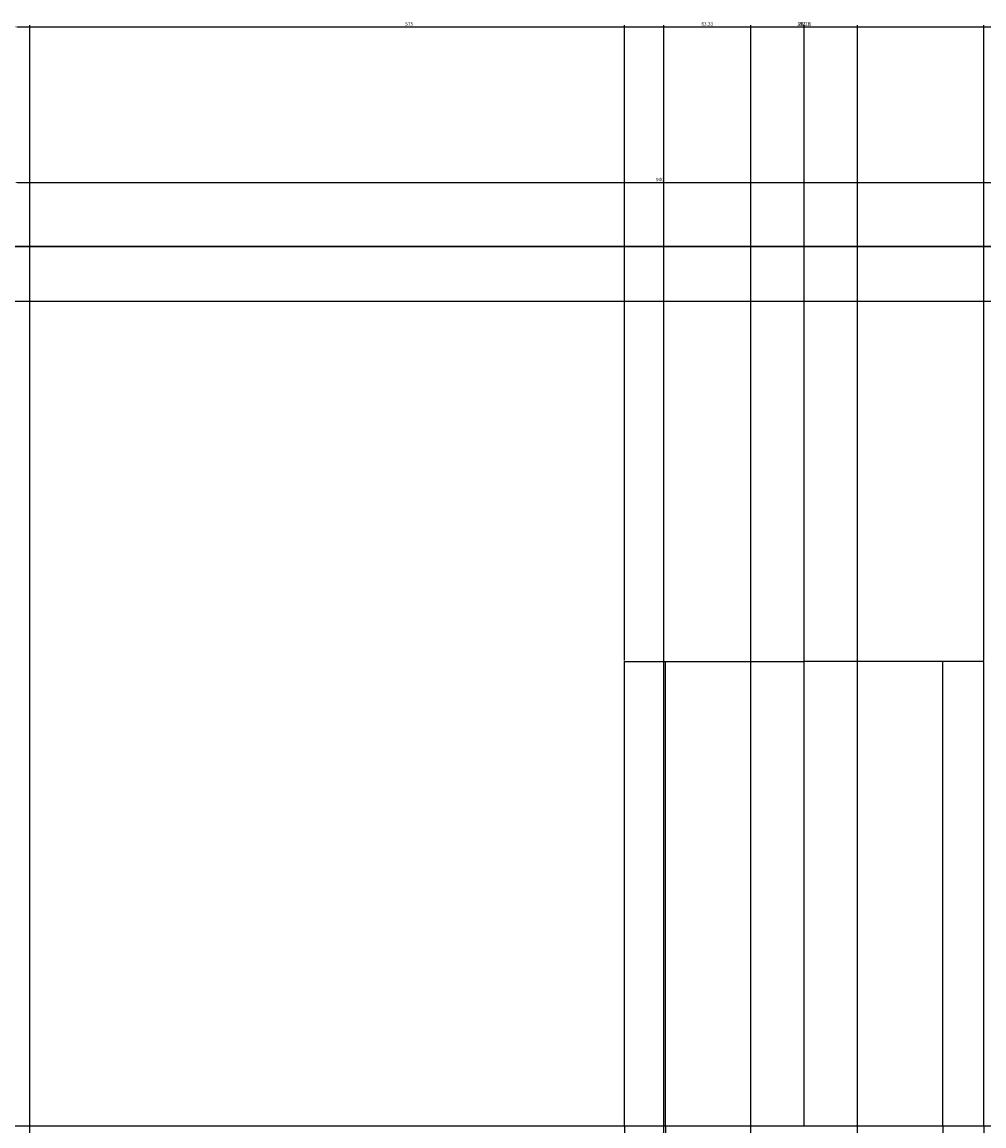
# Model space of a CAD drawing. Units: millimetres. Extents: x 2332 to 5836, y -853 to 2199.
# Tile 12 of 16: x 3641 to 4341, y 1368 to 2171. Entities that reach past the tile are written whole.
import ezdxf

# ---------------------------------------------------------------- set-up
doc = ezdxf.new("R2010")
doc.units = ezdxf.units.MM
for name, color, linetype, lineweight in [('A-ANNO-DIMS', 2, 'Continuous', 18), ('A-EQPM', 7, 'Continuous', 25), ('A-WALL', 8, 'Continuous', 30), ('SHELF', 40, 'Continuous', 25)]:
    doc.layers.add(name, color=color, linetype=linetype, lineweight=lineweight)
doc.styles.get("Standard").update_dxf_attribs({"font": 'arial.ttf'})
doc.dimstyles.new('ISO-25', dxfattribs={"dimtxt": 2.5, "dimasz": 2.5, "dimexe": 1.25, "dimexo": 0.625, "dimtad": 1, "dimtxsty": 'Standard', "dimcen": 2.5, "dimadec": 0, "dimazin": 0, "dimtfac": 1, "dimtmove": 0, "dimatfit": 3, "dimfxl": 1, "dimarcsym": 0})

# ---------------------------------------------------------------- blocks, each defined once
blk = doc.blocks.new('*D4')
at = {"layer": 'A-ANNO-DIMS', "color": 0, "lineweight": -2, "transparency": 16777216}
for p, q in [((3635.04, 2008.43), (3635.04, 2055.5)), ((3637.54, 2054.25), (4572.54, 2054.25)), ((4575.04, 2008.43), (4575.04, 2055.5))]:
    blk.add_line(p, q, dxfattribs=at)
at = {"layer": 'A-ANNO-DIMS', "color": 0, "transparency": 16777216}
for points in [[(3637.54, 2054.66), (3637.54, 2053.83), (3635.04, 2054.25)], [(4572.54, 2054.66), (4572.54, 2053.83), (4575.04, 2054.25)]]:
    blk.add_solid(points, dxfattribs=at)
at = {"layer": 'Defpoints', "color": 0, "transparency": 16777216}
for p in [(4575.04, 2054.25), (3635.04, 2007.8), (4575.04, 2007.8)]:
    blk.add_point(p, dxfattribs=at)
at = {"layer": 'A-ANNO-DIMS', "color": 0, "transparency": 16777216, "insert": (4105.04, 2056.15), "char_height": 2.5, "attachment_point": 5}
blk.add_mtext('940', dxfattribs=at)
blk = doc.blocks.new('*D23')
at = {"layer": 'A-ANNO-DIMS', "color": 0, "lineweight": -2, "transparency": 16777216}
for p, q in [((3646.47, 1030.43), (3646.47, 2168.7)), ((4773.61, 1030.43), (4773.61, 2168.7)), ((3648.97, 2167.45), (4771.11, 2167.45))]:
    blk.add_line(p, q, dxfattribs=at)
at = {"layer": 'A-ANNO-DIMS', "color": 0, "transparency": 16777216}
for points in [[(3648.97, 2167.87), (3648.97, 2167.04), (3646.47, 2167.45)], [(4771.11, 2167.87), (4771.11, 2167.04), (4773.61, 2167.45)]]:
    blk.add_solid(points, dxfattribs=at)
at = {"layer": 'Defpoints', "color": 0, "transparency": 16777216}
for p in [(4773.61, 2167.45), (3646.47, 1029.8), (4773.61, 1029.8)]:
    blk.add_point(p, dxfattribs=at)
at = {"layer": 'A-ANNO-DIMS', "color": 0, "transparency": 16777216, "insert": (4210.04, 2169.33), "char_height": 2.5, "attachment_point": 5}
blk.add_mtext('1127.1', dxfattribs=at)
blk = doc.blocks.new('*D24')
at = {"layer": 'A-ANNO-DIMS', "color": 0, "lineweight": -2, "transparency": 16777216}
for p, q in [((4079.19, 1706.43), (4079.19, 2168.7)), ((4340.89, 1706.43), (4340.89, 2168.7)), ((4081.69, 2167.45), (4338.39, 2167.45))]:
    blk.add_line(p, q, dxfattribs=at)
at = {"layer": 'A-ANNO-DIMS', "color": 0, "transparency": 16777216}
for points in [[(4081.69, 2167.87), (4081.69, 2167.04), (4079.19, 2167.45)], [(4338.39, 2167.87), (4338.39, 2167.04), (4340.89, 2167.45)]]:
    blk.add_solid(points, dxfattribs=at)
at = {"layer": 'Defpoints', "color": 0, "transparency": 16777216}
for p in [(4340.89, 2167.45), (4079.19, 1705.81), (4340.89, 1705.81)]:
    blk.add_point(p, dxfattribs=at)
at = {"layer": 'A-ANNO-DIMS', "color": 0, "transparency": 16777216, "insert": (4210.04, 2169.35), "char_height": 2.5, "attachment_point": 5}
blk.add_mtext('261.7', dxfattribs=at)
blk = doc.blocks.new('*D30')
at = {"layer": 'A-ANNO-DIMS', "color": 0, "lineweight": -2, "transparency": 16777216}
for p, q in [((3635.04, 1368.43), (3635.04, 2168.7)), ((4210.04, 1368.43), (4210.04, 2168.7)), ((3637.54, 2167.45), (4207.54, 2167.45))]:
    blk.add_line(p, q, dxfattribs=at)
at = {"layer": 'A-ANNO-DIMS', "color": 0, "transparency": 16777216}
for points in [[(3637.54, 2167.87), (3637.54, 2167.04), (3635.04, 2167.45)], [(4207.54, 2167.87), (4207.54, 2167.04), (4210.04, 2167.45)]]:
    blk.add_solid(points, dxfattribs=at)
at = {"layer": 'Defpoints', "color": 0, "transparency": 16777216}
for p in [(4210.04, 2167.45), (3635.04, 1367.8), (4210.04, 1367.8)]:
    blk.add_point(p, dxfattribs=at)
at = {"layer": 'A-ANNO-DIMS', "color": 0, "transparency": 16777216, "insert": (3922.54, 2169.35), "char_height": 2.5, "attachment_point": 5}
blk.add_mtext('575', dxfattribs=at)
blk = doc.blocks.new('*D31')
at = {"layer": 'A-ANNO-DIMS', "color": 0, "lineweight": -2, "transparency": 16777216}
for p, q in [((4171.16, 1017.67), (4171.16, 2168.7)), ((4248.92, 1017.67), (4248.92, 2168.7)), ((4173.66, 2167.45), (4246.42, 2167.45))]:
    blk.add_line(p, q, dxfattribs=at)
at = {"layer": 'A-ANNO-DIMS', "color": 0, "transparency": 16777216}
for points in [[(4173.66, 2167.87), (4173.66, 2167.04), (4171.16, 2167.45)], [(4246.42, 2167.87), (4246.42, 2167.04), (4248.92, 2167.45)]]:
    blk.add_solid(points, dxfattribs=at)
at = {"layer": 'Defpoints', "color": 0, "transparency": 16777216}
for p in [(4248.92, 2167.45), (4171.16, 1017.04), (4248.92, 1017.04)]:
    blk.add_point(p, dxfattribs=at)
at = {"layer": 'A-ANNO-DIMS', "color": 0, "transparency": 16777216, "insert": (4210.04, 2169.35), "char_height": 2.5, "attachment_point": 5}
blk.add_mtext('77.75', dxfattribs=at)
blk = doc.blocks.new('*D32')
at = {"layer": 'A-ANNO-DIMS', "color": 0, "lineweight": -2, "transparency": 16777216}
for p, q in [((4107.84, 1017.67), (4107.84, 2168.7)), ((4171.16, 1017.67), (4171.16, 2168.7)), ((4110.34, 2167.45), (4168.66, 2167.45))]:
    blk.add_line(p, q, dxfattribs=at)
at = {"layer": 'A-ANNO-DIMS', "color": 0, "transparency": 16777216}
for points in [[(4110.34, 2167.87), (4110.34, 2167.04), (4107.84, 2167.45)], [(4168.66, 2167.87), (4168.66, 2167.04), (4171.16, 2167.45)]]:
    blk.add_solid(points, dxfattribs=at)
at = {"layer": 'Defpoints', "color": 0, "transparency": 16777216}
for p in [(4171.16, 2167.45), (4107.84, 1017.04), (4171.16, 1017.04)]:
    blk.add_point(p, dxfattribs=at)
at = {"layer": 'A-ANNO-DIMS', "color": 0, "transparency": 16777216, "insert": (4139.5, 2169.36), "char_height": 2.5, "attachment_point": 5}
blk.add_mtext('63.33', dxfattribs=at)

msp = doc.modelspace()

# ---------------------------------------------------------------- linework, layer by layer
at = {"layer": 'A-EQPM'}
for p, q in [((4079.186, 1367.803), (4079.186, 1705.805)), ((4079.186, 1705.805), (4210.04, 1705.805)), ((4109.186, 1367.803), (4109.186, 1705.805)), ((4340.894, 1705.805), (4210.04, 1705.805)), ((4310.894, 1367.803), (4310.894, 1705.805)), ((4340.894, 1367.803), (4340.894, 1705.805)), ((4079.186, 1367.803), (4079.186, 1029.801)), ((4109.186, 1367.803), (4109.186, 1029.801)), ((4310.894, 1367.803), (4310.894, 1029.801)), ((4340.894, 1367.803), (4340.894, 1029.801))]:
    msp.add_line(p, q, dxfattribs=at)
at = {"layer": 'A-WALL'}
msp.add_line((3635.04, 2007.803), (4575.04, 2007.803), dxfattribs=at)
at = {"layer": 'SHELF'}
for p, q in [((3095.04, 1967.803), (4785.04, 1967.803)), ((4210.04, 1367.803), (4210.04, 1967.803)), ((3635.04, 1367.803), (4785.04, 1367.803))]:
    msp.add_line(p, q, dxfattribs=at)

# ---------------------------------------------------------------- dimensions: what is measured, and where the dimension line sits
at = {"layer": 'A-ANNO-DIMS'}
for base, p1, p2, override, picture, middle in [((4210.04, 2167.453), (3635.04, 1367.803), (4210.04, 1367.803), {"dimdec": 0, "dimlfac": 1, "dimrnd": 0, "dimzin": 0, "dimdsep": 46, "dimlunit": 2}, '*D30', (3922.54, 2169.35)), ((4773.612, 2167.453), (3646.468, 1029.801), (4773.612, 1029.801), {"dimdec": 1, "dimlfac": 1, "dimrnd": 0, "dimzin": 0, "dimdsep": 46, "dimlunit": 2}, '*D23', (4210.04, 2169.334)), ((4340.894, 2167.453), (4079.186, 1705.805), (4340.894, 1705.805), {"dimdec": 1, "dimlfac": 1, "dimrnd": 0, "dimzin": 0, "dimdsep": 46, "dimlunit": 2}, '*D24', (4210.04, 2169.355)), ((4171.163, 2167.453), (4107.837, 1017.045), (4171.163, 1017.045), {"dimdec": 2, "dimlfac": 1, "dimrnd": 0, "dimzin": 0, "dimdsep": 46, "dimlunit": 2}, '*D32', (4139.5, 2169.356)), ((4248.917, 2167.453), (4171.163, 1017.045), (4248.917, 1017.045), {"dimdec": 2, "dimlfac": 1, "dimrnd": 0, "dimzin": 0, "dimdsep": 46, "dimlunit": 2}, '*D31', (4210.04, 2169.35)), ((4575.04, 2054.248), (3635.04, 2007.803), (4575.04, 2007.803), {"dimclrd": 0, "dimclre": 0, "dimclrt": 0}, '*D4', (4105.04, 2056.149))]:
    dim = msp.add_linear_dim(base=base, p1=p1, p2=p2, dimstyle='ISO-25', override=override, dxfattribs=at)
    dim.commit()
    dim.dimension.update_dxf_attribs({"geometry": picture, "text_midpoint": middle})

doc.saveas('drawing.dxf')
